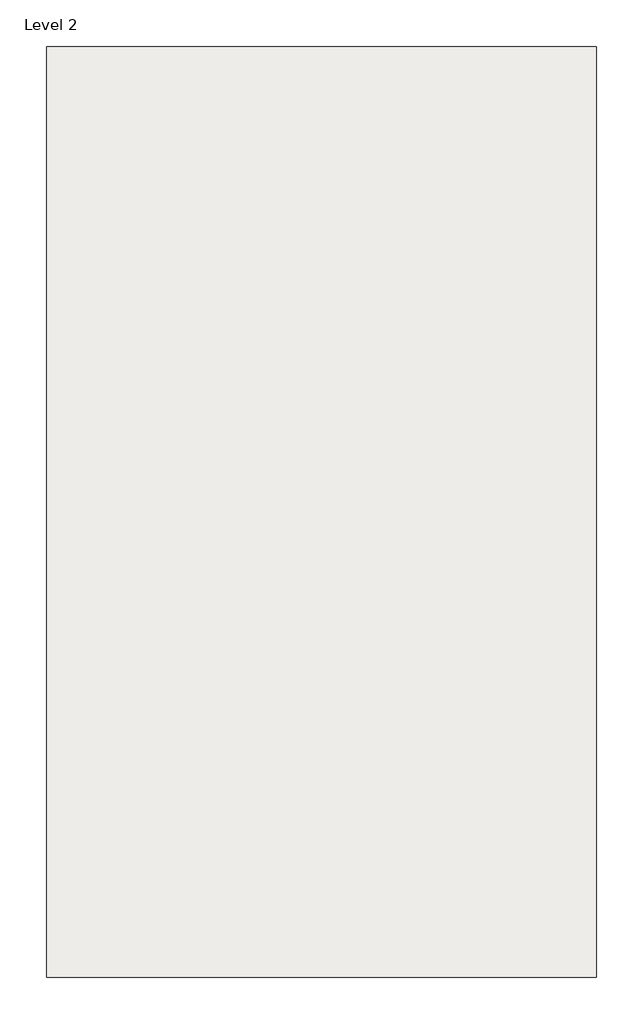
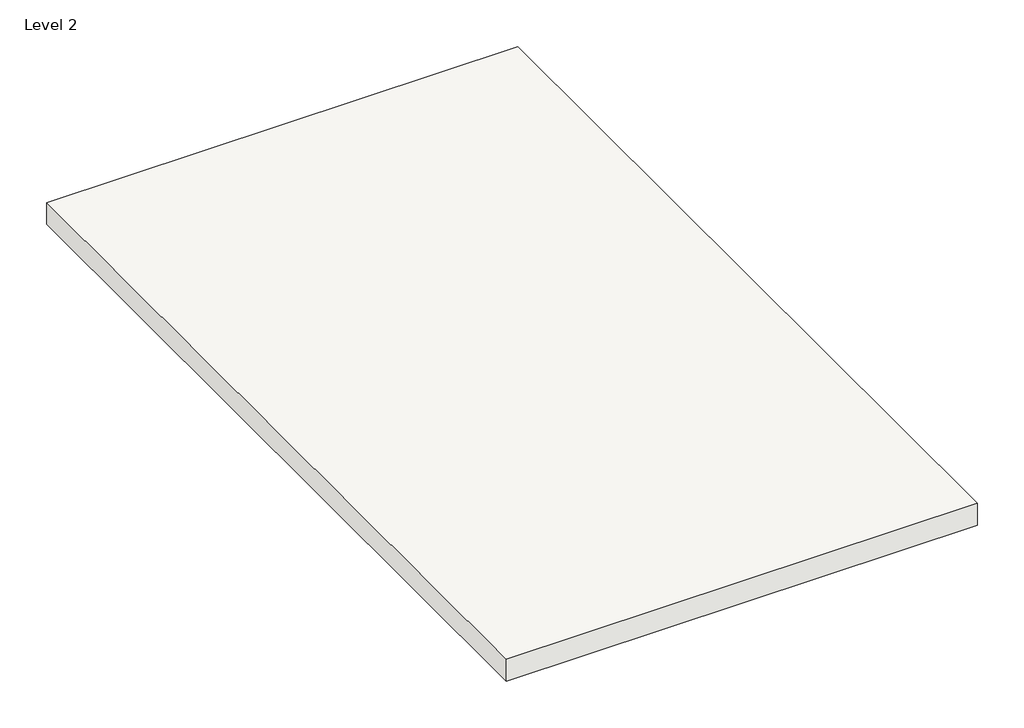
# One storey: 1 roof.
"""IFC4 building model written with IfcOpenShell, lengths in millimetres."""

from ifc_helpers import new_model, si_unit, frame, origin, place, context, project, spatial, polyline, outline, extrude, element, save

model = new_model("IFC4")

# Units and contexts
model_context = context("Model", 3, world=origin())
ifc_project = project(units=[si_unit("LENGTHUNIT", "METRE", prefix="MILLI")], contexts=[model_context])

# Site, building, storey
site = spatial("IfcSite", under=ifc_project)
building = spatial("IfcBuilding", under=site)
storey = spatial("IfcBuildingStorey", under=building, Name="Level 2", Elevation=3048.0)

# Roof
placement = place(None, origin())
element("IfcRoof", 1, ObjectType="Generic - 12\"", at=placement, inside=storey, context=model_context, shape_type="SweptSolid", body=[
    extrude(outline(polyline([(-16060.3757671, 16321.2418963), (-9761.1757671, 16321.2418963), (-9761.1757671, 5665.9418963), (-16060.3757671, 5665.9418963), (-16060.3757671, 16321.2418963)])), frame((0.0, 0.0, 3048.0), z_axis=(0.0, 0.0, 1.0), x_axis=(1.0, 0.0, 0.0)), (0.0, 0.0, 1.0), 304.8),
])

save(model, "model.ifc")

# Revit data of these elements
# Type "Generic - 12\""
#   Assembly Code = "B1020"
#   Layers, outside or top first: 1' - 0" "Brick, Soldier Course" (function 1)
# Element 1 (IfcRoof, "Generic - 12\"")
#   built-in parameter 1001705 = 11 (stored number, unit not read)
#   built-in parameter 1001710 = 33615
#   Phase Created = New Construction
#   Materials on its faces: "Brick, Soldier Course"
# Materials
#   "Brick, Soldier Course": class "Masonry", colour RGB 170 98 104, transparency 0, Description = "Common brick soldier coursed", Cost = 0
